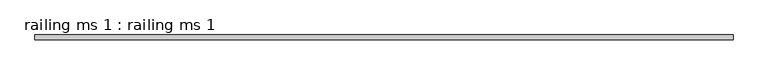
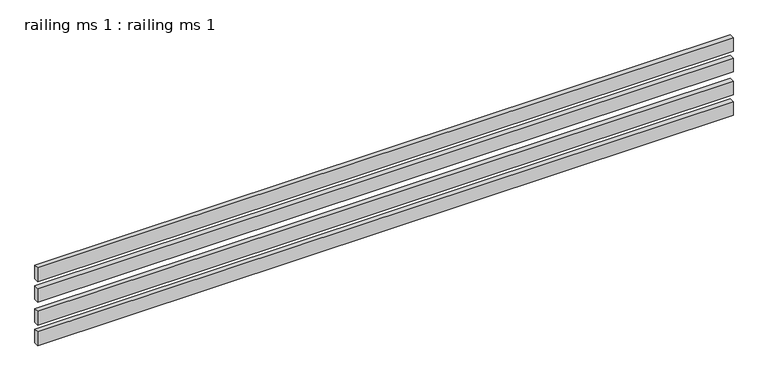
"""IFC4 building model written with IfcOpenShell, lengths in millimetres: proxy geometry, railing ms 1 : railing ms 1."""

from ifc_helpers import new_model, si_unit, frame, origin, place, context, project, spatial, polyline, outline, extrude, source, transform, mapped, element, save


def railing_ms_1_railing_ms_1_2379e55e(model_context):
    return source(origin(), model_context, "Body", "SweptSolid", [
        extrude(outline(polyline([(-15346.729089, -4413.5224035), (-15346.729089, -4438.9224035), (-19004.329089, -4438.9224035), (-19004.329089, -4413.5224035), (-15346.729089, -4413.5224035)])), frame((0.0, 0.0, 7052.1286522), z_axis=(0.0, 0.0, 1.0), x_axis=(1.0, 0.0, 0.0)), (0.0, 0.0, 1.0), 76.2),
        extrude(outline(polyline([(-15346.729089, -4413.5224035), (-15346.729089, -4438.9224035), (-19004.329089, -4438.9224035), (-19004.329089, -4413.5224035), (-15346.729089, -4413.5224035)])), frame((0.0, 0.0, 7166.4286522), z_axis=(0.0, 0.0, 1.0), x_axis=(1.0, 0.0, 0.0)), (0.0, 0.0, 1.0), 76.2),
        extrude(outline(polyline([(-15346.729089, -4413.5224035), (-15346.729089, -4438.9224035), (-19004.329089, -4438.9224035), (-19004.329089, -4413.5224035), (-15346.729089, -4413.5224035)])), frame((0.0, 0.0, 7293.4286522), z_axis=(0.0, 0.0, 1.0), x_axis=(1.0, 0.0, 0.0)), (0.0, 0.0, 1.0), 76.2),
        extrude(outline(polyline([(-15346.729089, -4413.5224035), (-15346.729089, -4438.9224035), (-19004.329089, -4438.9224035), (-19004.329089, -4413.5224035), (-15346.729089, -4413.5224035)])), frame((0.0, 0.0, 7407.7286522), z_axis=(0.0, 0.0, 1.0), x_axis=(1.0, 0.0, 0.0)), (0.0, 0.0, 1.0), 76.2),
    ])


if __name__ == "__main__":
    model = new_model("IFC4")
    model_context = context("Model", 3, world=origin())
    ifc_project = project(units=[si_unit("LENGTHUNIT", "METRE", prefix="MILLI")], contexts=[model_context])
    site = spatial("IfcSite", under=ifc_project)
    building = spatial("IfcBuilding", under=site)
    placement = place(None, origin())
    railing_ms_1_railing_ms_1_shape = railing_ms_1_railing_ms_1_2379e55e(model_context)
    element("IfcBuildingElementProxy", 1, Name="railing ms 1 : railing ms 1", ObjectType="railing ms 1 : railing ms 1", at=placement, inside=building, context=model_context, shape_type="MappedRepresentation", body=[
        mapped(railing_ms_1_railing_ms_1_shape, transform((0.0, 0.0, 0.0), x_axis=(1.0, 0.0, 0.0), y_axis=(0.0, 1.0, 0.0), z_axis=(0.0, 0.0, 1.0))),
    ])
    save(model, "model.ifc")
